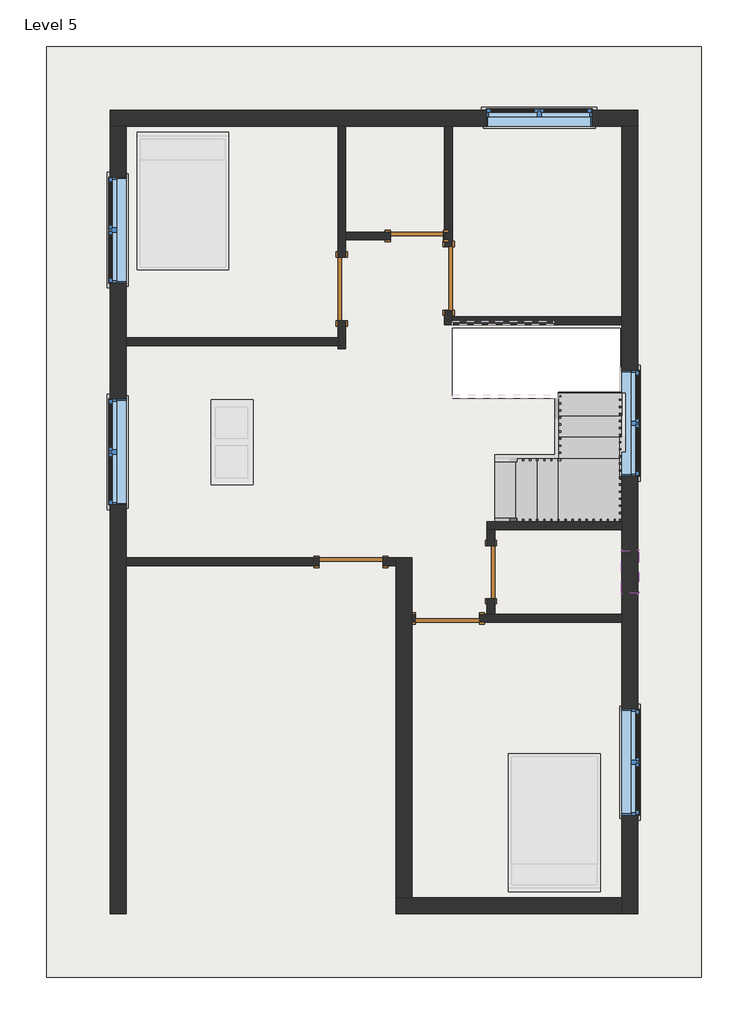
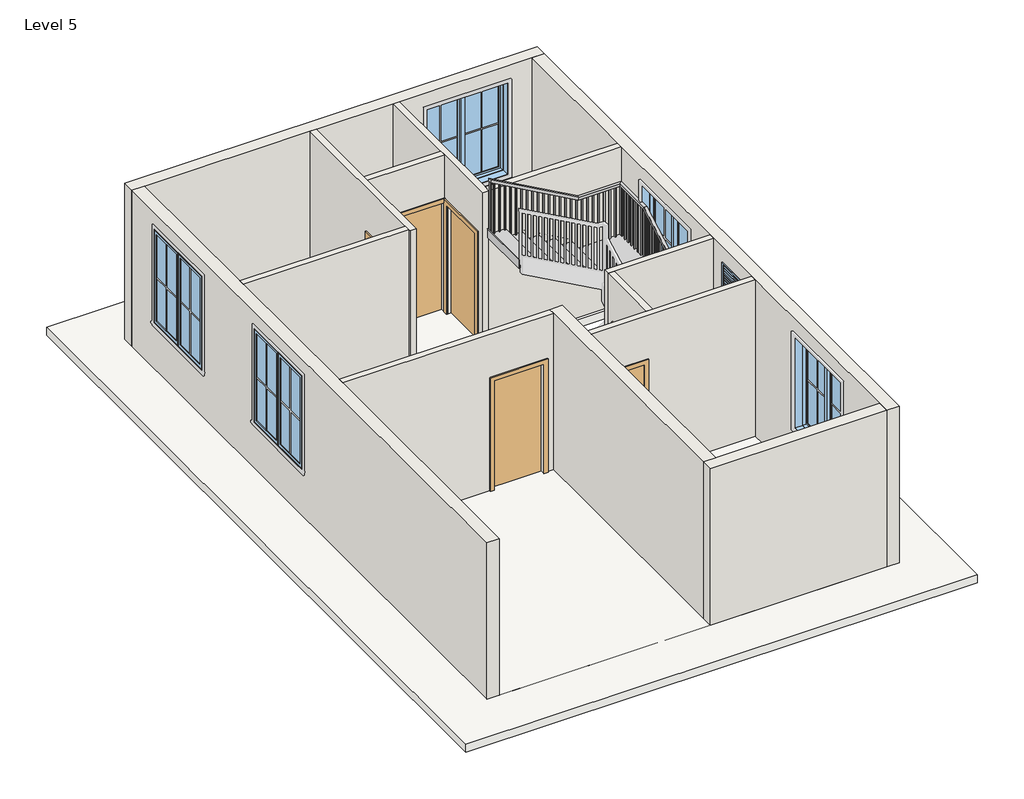
# One storey, part 1 of 2: 14 walls, 6 doors, 6 windows, 1 railing, 1 roof, 1 slab, 1 stair flight.
"""IFC4 building model written with IfcOpenShell, lengths in millimetres."""

from ifc_helpers import new_model, si_unit, frame, origin, place, context, project, spatial, polyline, outline, extrude, faceted_brep, transform, mapped, element, save
from components import door_214872d5, door_78caadf7, single_flush_door_3_e5f9f3c4, single_flush_door_3_305aa2a5, stair_flight_4ba9adf8, window_casement_double_win_5_f93960c7, window_f2d8fef0

model = new_model("IFC4")

# Units and contexts
model_context = context("Model", 3, world=origin())
ifc_project = project(units=[si_unit("LENGTHUNIT", "METRE", prefix="MILLI")], contexts=[model_context])

# Site, building, storey
site = spatial("IfcSite", under=ifc_project)
building = spatial("IfcBuilding", under=site)
storey = spatial("IfcBuildingStorey", under=building, Name="Level 5", Elevation=9601.2)

# Doors
placement = place(None, origin())
door_shape = door_214872d5(model_context)
element("IfcDoor", 1, ObjectType="Single-Flush : DOOR 2'6\"", at=placement, inside=storey, context=model_context, shape_type="MappedRepresentation", body=[
    mapped(door_shape, transform((-185.4325206, 3926.3629493, 9601.2), x_axis=(1.0, 0.0, 0.0), y_axis=(0.0, 1.0, 0.0), z_axis=(0.0, 0.0, 1.0))),
])
door_2_shape = door_78caadf7(model_context)
element("IfcDoor", 2, ObjectType="Single-Flush : DOOR 2'6\"", at=placement, inside=storey, context=model_context, shape_type="MappedRepresentation", body=[
    mapped(door_2_shape, transform((881.3674794, -905.9870507, 9601.2), x_axis=(0.0, 1.0, 0.0), y_axis=(-1.0, 0.0, 0.0), z_axis=(0.0, 0.0, 1.0))),
])
single_flush_door_3_shape = single_flush_door_3_e5f9f3c4(model_context)
element("IfcDoor", 3, ObjectType="Single-Flush : DOOR 3'", at=placement, inside=storey, context=model_context, shape_type="MappedRepresentation", body=[
    mapped(single_flush_door_3_shape, transform((271.7674794, 3316.7629493, 9601.2), x_axis=(0.0, -1.0, 0.0), y_axis=(1.0, 0.0, 0.0), z_axis=(0.0, 0.0, 1.0))),
])
element("IfcDoor", 4, ObjectType="Single-Flush : DOOR 3'", at=placement, inside=storey, context=model_context, shape_type="MappedRepresentation", body=[
    mapped(single_flush_door_3_shape, transform((255.8924794, -1572.7370507, 9601.2), x_axis=(-1.0, 0.0, 0.0), y_axis=(0.0, -1.0, 0.0), z_axis=(0.0, 0.0, 1.0))),
])
single_flush_door_3_2_shape = single_flush_door_3_305aa2a5(model_context)
element("IfcDoor", 5, ObjectType="Single-Flush : DOOR 3'", at=placement, inside=storey, context=model_context, shape_type="MappedRepresentation", body=[
    mapped(single_flush_door_3_2_shape, transform((-1264.9325206, 3164.3629493, 9601.2), x_axis=(0.0, -1.0, 0.0), y_axis=(1.0, 0.0, 0.0), z_axis=(0.0, 0.0, 1.0))),
])
element("IfcDoor", 6, ObjectType="Single-Flush : DOOR 3'6\"", at=placement, inside=storey, context=model_context, shape_type="MappedRepresentation", body=[
    mapped(single_flush_door_3_shape, transform((-1131.5825206, -759.9370507, 9601.2), x_axis=(1.0, 0.0, 0.0), y_axis=(0.0, 1.0, 0.0), z_axis=(0.0, 0.0, 1.0))),
])

# Railing
element("IfcRailing", 7, ObjectType="Handrail - Rectangular", at=placement, inside=storey, context=model_context, shape_type="SolidModel", body=[
    faceted_brep([(938.5174794, -131.2870507, 10684.9333333), (938.5174794, -131.2870507, 10626.820221), (938.5174794, -182.0870507, 10626.820221), (938.5174794, -182.0870507, 10684.9333333), (2005.3174794, -131.2870507, 11277.6), (2018.4810817, -131.2870507, 11226.8), (2018.4810817, -182.0870507, 11226.8), (2005.3174794, -182.0870507, 11277.6), (2716.5174794, -131.2870507, 11277.6), (2716.5174794, -131.2870507, 11226.8), (2767.3174794, -182.0870507, 11226.8), (2767.3174794, -182.0870507, 11277.6), (2716.5174794, 579.9129493, 11277.6), (2716.5174794, 593.0765516, 11226.8), (2767.3174794, 593.0765516, 11226.8), (2767.3174794, 579.9129493, 11277.6), (2716.5174794, 1843.5629493, 11979.6277778), (2716.5174794, 1856.7265516, 11928.8277778), (2767.3174794, 1856.7265516, 11928.8277778), (2767.3174794, 1843.5629493, 11979.6277778), (2716.5174794, 2599.2129493, 11979.6277778), (2716.5174794, 2599.2129493, 11928.8277778), (2767.3174794, 2650.0129493, 11928.8277778), (2767.3174794, 2650.0129493, 11979.6277778), (1960.8674794, 2599.2129493, 11979.6277778), (1947.7038772, 2599.2129493, 11928.8277778), (1947.7038772, 2650.0129493, 11928.8277778), (1960.8674794, 2650.0129493, 11979.6277778), (328.9174794, 2599.2129493, 12886.2666667), (328.9174794, 2650.0129493, 12886.2666667), (328.9174794, 2650.0129493, 12828.1535543), (328.9174794, 2599.2129493, 12828.1535543)], [[[0, 1, 2, 3]], [[1, 0, 4, 5]], [[2, 1, 5, 6]], [[3, 2, 6, 7]], [[0, 3, 7, 4]], [[5, 4, 8, 9]], [[6, 5, 9, 10]], [[7, 6, 10, 11]], [[4, 7, 11, 8]], [[9, 8, 12, 13]], [[10, 9, 13, 14]], [[11, 10, 14, 15]], [[8, 11, 15, 12]], [[13, 12, 16, 17]], [[14, 13, 17, 18]], [[15, 14, 18, 19]], [[12, 15, 19, 16]], [[17, 16, 20, 21]], [[18, 17, 21, 22]], [[19, 18, 22, 23]], [[16, 19, 23, 20]], [[21, 20, 24, 25]], [[22, 21, 25, 26]], [[23, 22, 26, 27]], [[20, 23, 27, 24]], [[28, 29, 30, 31]], [[25, 24, 28, 31]], [[26, 25, 31, 30]], [[27, 26, 30, 29]], [[24, 27, 29, 28]]]),
    extrude(outline(polyline([(12780.5285543, 414.6424794), (12791.1118876, 395.5924794), (11802.5333333, 395.5924794), (11802.5333333, 414.6424794), (12780.5285543, 414.6424794)])), frame((0.0, 2615.0879493, 0.0), z_axis=(0.0, 1.0, 0.0), x_axis=(0.0, 0.0, 1.0)), (0.0, 0.0, 1.0), 19.05),
    extrude(outline(polyline([(12724.0841099, 516.2424794), (12734.6674432, 497.1924794), (11802.5333333, 497.1924794), (11802.5333333, 516.2424794), (12724.0841099, 516.2424794)])), frame((0.0, 2615.0879493, 0.0), z_axis=(0.0, 1.0, 0.0), x_axis=(0.0, 0.0, 1.0)), (0.0, 0.0, 1.0), 19.05),
    extrude(outline(polyline([(12667.6396654, 617.8424794), (12678.2229988, 598.7924794), (11802.5333333, 598.7924794), (11802.5333333, 617.8424794), (12667.6396654, 617.8424794)])), frame((0.0, 2615.0879493, 0.0), z_axis=(0.0, 1.0, 0.0), x_axis=(0.0, 0.0, 1.0)), (0.0, 0.0, 1.0), 19.05),
    extrude(outline(polyline([(12611.195221, 719.4424794), (12621.7785543, 700.3924794), (11633.2, 700.3924794), (11633.2, 719.4424794), (12611.195221, 719.4424794)])), frame((0.0, 2615.0879493, 0.0), z_axis=(0.0, 1.0, 0.0), x_axis=(0.0, 0.0, 1.0)), (0.0, 0.0, 1.0), 19.05),
    extrude(outline(polyline([(12554.7507765, 821.0424794), (12565.3341099, 801.9924794), (11633.2, 801.9924794), (11633.2, 821.0424794), (12554.7507765, 821.0424794)])), frame((0.0, 2615.0879493, 0.0), z_axis=(0.0, 1.0, 0.0), x_axis=(0.0, 0.0, 1.0)), (0.0, 0.0, 1.0), 19.05),
    extrude(outline(polyline([(12498.3063321, 922.6424794), (12508.8896654, 903.5924794), (11633.2, 903.5924794), (11633.2, 922.6424794), (12498.3063321, 922.6424794)])), frame((0.0, 2615.0879493, 0.0), z_axis=(0.0, 1.0, 0.0), x_axis=(0.0, 0.0, 1.0)), (0.0, 0.0, 1.0), 19.05),
    extrude(outline(polyline([(12441.8618876, 1024.2424794), (12452.445221, 1005.1924794), (11463.8666667, 1005.1924794), (11463.8666667, 1024.2424794), (12441.8618876, 1024.2424794)])), frame((0.0, 2615.0879493, 0.0), z_axis=(0.0, 1.0, 0.0), x_axis=(0.0, 0.0, 1.0)), (0.0, 0.0, 1.0), 19.05),
    extrude(outline(polyline([(12385.4174432, 1125.8424794), (12396.0007765, 1106.7924794), (11463.8666667, 1106.7924794), (11463.8666667, 1125.8424794), (12385.4174432, 1125.8424794)])), frame((0.0, 2615.0879493, 0.0), z_axis=(0.0, 1.0, 0.0), x_axis=(0.0, 0.0, 1.0)), (0.0, 0.0, 1.0), 19.05),
    extrude(outline(polyline([(12328.9729988, 1227.4424794), (12339.5563321, 1208.3924794), (11463.8666667, 1208.3924794), (11463.8666667, 1227.4424794), (12328.9729988, 1227.4424794)])), frame((0.0, 2615.0879493, 0.0), z_axis=(0.0, 1.0, 0.0), x_axis=(0.0, 0.0, 1.0)), (0.0, 0.0, 1.0), 19.05),
    extrude(outline(polyline([(12272.5285543, 1329.0424794), (12283.1118876, 1309.9924794), (11294.5333333, 1309.9924794), (11294.5333333, 1329.0424794), (12272.5285543, 1329.0424794)])), frame((0.0, 2615.0879493, 0.0), z_axis=(0.0, 1.0, 0.0), x_axis=(0.0, 0.0, 1.0)), (0.0, 0.0, 1.0), 19.05),
    extrude(outline(polyline([(12216.0841099, 1430.6424794), (12226.6674432, 1411.5924794), (11294.5333333, 1411.5924794), (11294.5333333, 1430.6424794), (12216.0841099, 1430.6424794)])), frame((0.0, 2615.0879493, 0.0), z_axis=(0.0, 1.0, 0.0), x_axis=(0.0, 0.0, 1.0)), (0.0, 0.0, 1.0), 19.05),
    extrude(outline(polyline([(12159.6396654, 1532.2424794), (12170.2229988, 1513.1924794), (11294.5333333, 1513.1924794), (11294.5333333, 1532.2424794), (12159.6396654, 1532.2424794)])), frame((0.0, 2615.0879493, 0.0), z_axis=(0.0, 1.0, 0.0), x_axis=(0.0, 0.0, 1.0)), (0.0, 0.0, 1.0), 19.05),
    extrude(outline(polyline([(12103.195221, 1633.8424794), (12113.7785543, 1614.7924794), (11125.2, 1614.7924794), (11125.2, 1633.8424794), (12103.195221, 1633.8424794)])), frame((0.0, 2615.0879493, 0.0), z_axis=(0.0, 1.0, 0.0), x_axis=(0.0, 0.0, 1.0)), (0.0, 0.0, 1.0), 19.05),
    extrude(outline(polyline([(12046.7507765, 1735.4424794), (12057.3341099, 1716.3924794), (11125.2, 1716.3924794), (11125.2, 1735.4424794), (12046.7507765, 1735.4424794)])), frame((0.0, 2615.0879493, 0.0), z_axis=(0.0, 1.0, 0.0), x_axis=(0.0, 0.0, 1.0)), (0.0, 0.0, 1.0), 19.05),
    extrude(outline(polyline([(11990.3063321, 1837.0424794), (12000.8896654, 1817.9924794), (11125.2, 1817.9924794), (11125.2, 1837.0424794), (11990.3063321, 1837.0424794)])), frame((0.0, 2615.0879493, 0.0), z_axis=(0.0, 1.0, 0.0), x_axis=(0.0, 0.0, 1.0)), (0.0, 0.0, 1.0), 19.05),
    extrude(outline(polyline([(11933.8618876, 1938.6424794), (11944.445221, 1919.5924794), (10955.8666667, 1919.5924794), (10955.8666667, 1938.6424794), (11933.8618876, 1938.6424794)])), frame((0.0, 2615.0879493, 0.0), z_axis=(0.0, 1.0, 0.0), x_axis=(0.0, 0.0, 1.0)), (0.0, 0.0, 1.0), 19.05),
    extrude(outline(polyline([(2040.2424794, 2634.1379493), (2040.2424794, 2615.0879493), (2021.1924794, 2615.0879493), (2021.1924794, 2634.1379493), (2040.2424794, 2634.1379493)])), frame((0.0, 0.0, 10955.8666667), z_axis=(0.0, 0.0, 1.0), x_axis=(1.0, 0.0, 0.0)), (0.0, 0.0, 1.0), 972.9611111),
    extrude(outline(polyline([(2141.8424794, 2634.1379493), (2141.8424794, 2615.0879493), (2122.7924794, 2615.0879493), (2122.7924794, 2634.1379493), (2141.8424794, 2634.1379493)])), frame((0.0, 0.0, 10955.8666667), z_axis=(0.0, 0.0, 1.0), x_axis=(1.0, 0.0, 0.0)), (0.0, 0.0, 1.0), 972.9611111),
    extrude(outline(polyline([(2243.4424794, 2634.1379493), (2243.4424794, 2615.0879493), (2224.3924794, 2615.0879493), (2224.3924794, 2634.1379493), (2243.4424794, 2634.1379493)])), frame((0.0, 0.0, 10955.8666667), z_axis=(0.0, 0.0, 1.0), x_axis=(1.0, 0.0, 0.0)), (0.0, 0.0, 1.0), 972.9611111),
    extrude(outline(polyline([(2345.0424794, 2634.1379493), (2345.0424794, 2615.0879493), (2325.9924794, 2615.0879493), (2325.9924794, 2634.1379493), (2345.0424794, 2634.1379493)])), frame((0.0, 0.0, 10955.8666667), z_axis=(0.0, 0.0, 1.0), x_axis=(1.0, 0.0, 0.0)), (0.0, 0.0, 1.0), 972.9611111),
    extrude(outline(polyline([(2446.6424794, 2634.1379493), (2446.6424794, 2615.0879493), (2427.5924794, 2615.0879493), (2427.5924794, 2634.1379493), (2446.6424794, 2634.1379493)])), frame((0.0, 0.0, 10955.8666667), z_axis=(0.0, 0.0, 1.0), x_axis=(1.0, 0.0, 0.0)), (0.0, 0.0, 1.0), 972.9611111),
    extrude(outline(polyline([(2548.2424794, 2634.1379493), (2548.2424794, 2615.0879493), (2529.1924794, 2615.0879493), (2529.1924794, 2634.1379493), (2548.2424794, 2634.1379493)])), frame((0.0, 0.0, 10955.8666667), z_axis=(0.0, 0.0, 1.0), x_axis=(1.0, 0.0, 0.0)), (0.0, 0.0, 1.0), 972.9611111),
    extrude(outline(polyline([(2649.8424794, 2634.1379493), (2649.8424794, 2615.0879493), (2630.7924794, 2615.0879493), (2630.7924794, 2634.1379493), (2649.8424794, 2634.1379493)])), frame((0.0, 0.0, 10955.8666667), z_axis=(0.0, 0.0, 1.0), x_axis=(1.0, 0.0, 0.0)), (0.0, 0.0, 1.0), 972.9611111),
    extrude(outline(polyline([(2751.4424794, 2576.9879493), (2732.3924794, 2576.9879493), (2732.3924794, 2596.0379493), (2751.4424794, 2596.0379493), (2751.4424794, 2576.9879493)])), frame((0.0, 0.0, 10955.8666667), z_axis=(0.0, 0.0, 1.0), x_axis=(1.0, 0.0, 0.0)), (0.0, 0.0, 1.0), 972.9611111),
    extrude(outline(polyline([(2751.4424794, 2475.3879493), (2732.3924794, 2475.3879493), (2732.3924794, 2494.4379493), (2751.4424794, 2494.4379493), (2751.4424794, 2475.3879493)])), frame((0.0, 0.0, 10955.8666667), z_axis=(0.0, 0.0, 1.0), x_axis=(1.0, 0.0, 0.0)), (0.0, 0.0, 1.0), 972.9611111),
    extrude(outline(polyline([(2751.4424794, 2373.7879493), (2732.3924794, 2373.7879493), (2732.3924794, 2392.8379493), (2751.4424794, 2392.8379493), (2751.4424794, 2373.7879493)])), frame((0.0, 0.0, 10955.8666667), z_axis=(0.0, 0.0, 1.0), x_axis=(1.0, 0.0, 0.0)), (0.0, 0.0, 1.0), 972.9611111),
    extrude(outline(polyline([(2751.4424794, 2272.1879493), (2732.3924794, 2272.1879493), (2732.3924794, 2291.2379493), (2751.4424794, 2291.2379493), (2751.4424794, 2272.1879493)])), frame((0.0, 0.0, 10955.8666667), z_axis=(0.0, 0.0, 1.0), x_axis=(1.0, 0.0, 0.0)), (0.0, 0.0, 1.0), 972.9611111),
    extrude(outline(polyline([(2751.4424794, 2170.5879493), (2732.3924794, 2170.5879493), (2732.3924794, 2189.6379493), (2751.4424794, 2189.6379493), (2751.4424794, 2170.5879493)])), frame((0.0, 0.0, 10955.8666667), z_axis=(0.0, 0.0, 1.0), x_axis=(1.0, 0.0, 0.0)), (0.0, 0.0, 1.0), 972.9611111),
    extrude(outline(polyline([(2751.4424794, 2068.9879493), (2732.3924794, 2068.9879493), (2732.3924794, 2088.0379493), (2751.4424794, 2088.0379493), (2751.4424794, 2068.9879493)])), frame((0.0, 0.0, 10955.8666667), z_axis=(0.0, 0.0, 1.0), x_axis=(1.0, 0.0, 0.0)), (0.0, 0.0, 1.0), 972.9611111),
    extrude(outline(polyline([(2751.4424794, 1967.3879493), (2732.3924794, 1967.3879493), (2732.3924794, 1986.4379493), (2751.4424794, 1986.4379493), (2751.4424794, 1967.3879493)])), frame((0.0, 0.0, 10955.8666667), z_axis=(0.0, 0.0, 1.0), x_axis=(1.0, 0.0, 0.0)), (0.0, 0.0, 1.0), 972.9611111),
    extrude(outline(polyline([(2751.4424794, 1865.7879493), (2732.3924794, 1865.7879493), (2732.3924794, 1884.8379493), (2751.4424794, 1884.8379493), (2751.4424794, 1865.7879493)])), frame((0.0, 0.0, 10955.8666667), z_axis=(0.0, 0.0, 1.0), x_axis=(1.0, 0.0, 0.0)), (0.0, 0.0, 1.0), 972.9611111),
    extrude(outline(polyline([(1764.1879493, 11877.4174432), (1783.2379493, 11888.0007765), (1783.2379493, 10955.8666667), (1764.1879493, 10955.8666667), (1764.1879493, 11877.4174432)])), frame((2732.3924794, 0.0, 0.0), z_axis=(1.0, 0.0, 0.0), x_axis=(0.0, 1.0, 0.0)), (0.0, 0.0, 1.0), 19.05),
    extrude(outline(polyline([(1662.5879493, 11820.9729988), (1681.6379493, 11831.5563321), (1681.6379493, 10955.8666667), (1662.5879493, 10955.8666667), (1662.5879493, 11820.9729988)])), frame((2732.3924794, 0.0, 0.0), z_axis=(1.0, 0.0, 0.0), x_axis=(0.0, 1.0, 0.0)), (0.0, 0.0, 1.0), 19.05),
    extrude(outline(polyline([(1560.9879493, 11764.5285543), (1580.0379493, 11775.1118876), (1580.0379493, 10786.5333333), (1560.9879493, 10786.5333333), (1560.9879493, 11764.5285543)])), frame((2732.3924794, 0.0, 0.0), z_axis=(1.0, 0.0, 0.0), x_axis=(0.0, 1.0, 0.0)), (0.0, 0.0, 1.0), 19.05),
    extrude(outline(polyline([(1459.3879493, 11708.0841099), (1478.4379493, 11718.6674432), (1478.4379493, 10786.5333333), (1459.3879493, 10786.5333333), (1459.3879493, 11708.0841099)])), frame((2732.3924794, 0.0, 0.0), z_axis=(1.0, 0.0, 0.0), x_axis=(0.0, 1.0, 0.0)), (0.0, 0.0, 1.0), 19.05),
    extrude(outline(polyline([(1357.7879493, 11651.6396654), (1376.8379493, 11662.2229988), (1376.8379493, 10786.5333333), (1357.7879493, 10786.5333333), (1357.7879493, 11651.6396654)])), frame((2732.3924794, 0.0, 0.0), z_axis=(1.0, 0.0, 0.0), x_axis=(0.0, 1.0, 0.0)), (0.0, 0.0, 1.0), 19.05),
    extrude(outline(polyline([(1256.1879493, 11595.195221), (1275.2379493, 11605.7785543), (1275.2379493, 10617.2), (1256.1879493, 10617.2), (1256.1879493, 11595.195221)])), frame((2732.3924794, 0.0, 0.0), z_axis=(1.0, 0.0, 0.0), x_axis=(0.0, 1.0, 0.0)), (0.0, 0.0, 1.0), 19.05),
    extrude(outline(polyline([(1154.5879493, 11538.7507765), (1173.6379493, 11549.3341099), (1173.6379493, 10617.2), (1154.5879493, 10617.2), (1154.5879493, 11538.7507765)])), frame((2732.3924794, 0.0, 0.0), z_axis=(1.0, 0.0, 0.0), x_axis=(0.0, 1.0, 0.0)), (0.0, 0.0, 1.0), 19.05),
    extrude(outline(polyline([(1052.9879493, 11482.3063321), (1072.0379493, 11492.8896654), (1072.0379493, 10617.2), (1052.9879493, 10617.2), (1052.9879493, 11482.3063321)])), frame((2732.3924794, 0.0, 0.0), z_axis=(1.0, 0.0, 0.0), x_axis=(0.0, 1.0, 0.0)), (0.0, 0.0, 1.0), 19.05),
    extrude(outline(polyline([(951.3879493, 11425.8618876), (970.4379493, 11436.445221), (970.4379493, 10447.8666667), (951.3879493, 10447.8666667), (951.3879493, 11425.8618876)])), frame((2732.3924794, 0.0, 0.0), z_axis=(1.0, 0.0, 0.0), x_axis=(0.0, 1.0, 0.0)), (0.0, 0.0, 1.0), 19.05),
    extrude(outline(polyline([(849.7879493, 11369.4174432), (868.8379493, 11380.0007765), (868.8379493, 10447.8666667), (849.7879493, 10447.8666667), (849.7879493, 11369.4174432)])), frame((2732.3924794, 0.0, 0.0), z_axis=(1.0, 0.0, 0.0), x_axis=(0.0, 1.0, 0.0)), (0.0, 0.0, 1.0), 19.05),
    extrude(outline(polyline([(748.1879493, 11312.9729988), (767.2379493, 11323.5563321), (767.2379493, 10447.8666667), (748.1879493, 10447.8666667), (748.1879493, 11312.9729988)])), frame((2732.3924794, 0.0, 0.0), z_axis=(1.0, 0.0, 0.0), x_axis=(0.0, 1.0, 0.0)), (0.0, 0.0, 1.0), 19.05),
    extrude(outline(polyline([(646.5879493, 11256.5285543), (665.6379493, 11267.1118876), (665.6379493, 10278.5333333), (646.5879493, 10278.5333333), (646.5879493, 11256.5285543)])), frame((2732.3924794, 0.0, 0.0), z_axis=(1.0, 0.0, 0.0), x_axis=(0.0, 1.0, 0.0)), (0.0, 0.0, 1.0), 19.05),
    extrude(outline(polyline([(2751.4424794, 544.9879493), (2732.3924794, 544.9879493), (2732.3924794, 564.0379493), (2751.4424794, 564.0379493), (2751.4424794, 544.9879493)])), frame((0.0, 0.0, 10278.5333333), z_axis=(0.0, 0.0, 1.0), x_axis=(1.0, 0.0, 0.0)), (0.0, 0.0, 1.0), 948.2666667),
    extrude(outline(polyline([(2751.4424794, 443.3879493), (2732.3924794, 443.3879493), (2732.3924794, 462.4379493), (2751.4424794, 462.4379493), (2751.4424794, 443.3879493)])), frame((0.0, 0.0, 10278.5333333), z_axis=(0.0, 0.0, 1.0), x_axis=(1.0, 0.0, 0.0)), (0.0, 0.0, 1.0), 948.2666667),
    extrude(outline(polyline([(2751.4424794, 341.7879493), (2732.3924794, 341.7879493), (2732.3924794, 360.8379493), (2751.4424794, 360.8379493), (2751.4424794, 341.7879493)])), frame((0.0, 0.0, 10278.5333333), z_axis=(0.0, 0.0, 1.0), x_axis=(1.0, 0.0, 0.0)), (0.0, 0.0, 1.0), 948.2666667),
    extrude(outline(polyline([(2751.4424794, 240.1879493), (2732.3924794, 240.1879493), (2732.3924794, 259.2379493), (2751.4424794, 259.2379493), (2751.4424794, 240.1879493)])), frame((0.0, 0.0, 10278.5333333), z_axis=(0.0, 0.0, 1.0), x_axis=(1.0, 0.0, 0.0)), (0.0, 0.0, 1.0), 948.2666667),
    extrude(outline(polyline([(2751.4424794, 138.5879493), (2732.3924794, 138.5879493), (2732.3924794, 157.6379493), (2751.4424794, 157.6379493), (2751.4424794, 138.5879493)])), frame((0.0, 0.0, 10278.5333333), z_axis=(0.0, 0.0, 1.0), x_axis=(1.0, 0.0, 0.0)), (0.0, 0.0, 1.0), 948.2666667),
    extrude(outline(polyline([(2751.4424794, 36.9879493), (2732.3924794, 36.9879493), (2732.3924794, 56.0379493), (2751.4424794, 56.0379493), (2751.4424794, 36.9879493)])), frame((0.0, 0.0, 10278.5333333), z_axis=(0.0, 0.0, 1.0), x_axis=(1.0, 0.0, 0.0)), (0.0, 0.0, 1.0), 948.2666667),
    extrude(outline(polyline([(2751.4424794, -64.6120507), (2732.3924794, -64.6120507), (2732.3924794, -45.5620507), (2751.4424794, -45.5620507), (2751.4424794, -64.6120507)])), frame((0.0, 0.0, 10278.5333333), z_axis=(0.0, 0.0, 1.0), x_axis=(1.0, 0.0, 0.0)), (0.0, 0.0, 1.0), 948.2666667),
    extrude(outline(polyline([(2656.1924794, -166.2120507), (2656.1924794, -147.1620507), (2675.2424794, -147.1620507), (2675.2424794, -166.2120507), (2656.1924794, -166.2120507)])), frame((0.0, 0.0, 10278.5333333), z_axis=(0.0, 0.0, 1.0), x_axis=(1.0, 0.0, 0.0)), (0.0, 0.0, 1.0), 948.2666667),
    extrude(outline(polyline([(2554.5924794, -166.2120507), (2554.5924794, -147.1620507), (2573.6424794, -147.1620507), (2573.6424794, -166.2120507), (2554.5924794, -166.2120507)])), frame((0.0, 0.0, 10278.5333333), z_axis=(0.0, 0.0, 1.0), x_axis=(1.0, 0.0, 0.0)), (0.0, 0.0, 1.0), 948.2666667),
    extrude(outline(polyline([(2452.9924794, -166.2120507), (2452.9924794, -147.1620507), (2472.0424794, -147.1620507), (2472.0424794, -166.2120507), (2452.9924794, -166.2120507)])), frame((0.0, 0.0, 10278.5333333), z_axis=(0.0, 0.0, 1.0), x_axis=(1.0, 0.0, 0.0)), (0.0, 0.0, 1.0), 948.2666667),
    extrude(outline(polyline([(2351.3924794, -166.2120507), (2351.3924794, -147.1620507), (2370.4424794, -147.1620507), (2370.4424794, -166.2120507), (2351.3924794, -166.2120507)])), frame((0.0, 0.0, 10278.5333333), z_axis=(0.0, 0.0, 1.0), x_axis=(1.0, 0.0, 0.0)), (0.0, 0.0, 1.0), 948.2666667),
    extrude(outline(polyline([(2249.7924794, -166.2120507), (2249.7924794, -147.1620507), (2268.8424794, -147.1620507), (2268.8424794, -166.2120507), (2249.7924794, -166.2120507)])), frame((0.0, 0.0, 10278.5333333), z_axis=(0.0, 0.0, 1.0), x_axis=(1.0, 0.0, 0.0)), (0.0, 0.0, 1.0), 948.2666667),
    extrude(outline(polyline([(2148.1924794, -166.2120507), (2148.1924794, -147.1620507), (2167.2424794, -147.1620507), (2167.2424794, -166.2120507), (2148.1924794, -166.2120507)])), frame((0.0, 0.0, 10278.5333333), z_axis=(0.0, 0.0, 1.0), x_axis=(1.0, 0.0, 0.0)), (0.0, 0.0, 1.0), 948.2666667),
    extrude(outline(polyline([(2046.5924794, -166.2120507), (2046.5924794, -147.1620507), (2065.6424794, -147.1620507), (2065.6424794, -166.2120507), (2046.5924794, -166.2120507)])), frame((0.0, 0.0, 10278.5333333), z_axis=(0.0, 0.0, 1.0), x_axis=(1.0, 0.0, 0.0)), (0.0, 0.0, 1.0), 948.2666667),
    extrude(outline(polyline([(11196.5563321, 1964.0424794), (11185.9729988, 1944.9924794), (10278.5333333, 1944.9924794), (10278.5333333, 1964.0424794), (11196.5563321, 1964.0424794)])), frame((0.0, -166.2120507, 0.0), z_axis=(0.0, 1.0, 0.0), x_axis=(0.0, 0.0, 1.0)), (0.0, 0.0, 1.0), 19.05),
    extrude(outline(polyline([(11140.1118876, 1862.4424794), (11129.5285543, 1843.3924794), (10278.5333333, 1843.3924794), (10278.5333333, 1862.4424794), (11140.1118876, 1862.4424794)])), frame((0.0, -166.2120507, 0.0), z_axis=(0.0, 1.0, 0.0), x_axis=(0.0, 0.0, 1.0)), (0.0, 0.0, 1.0), 19.05),
    extrude(outline(polyline([(11083.6674432, 1760.8424794), (11073.0841099, 1741.7924794), (10109.2, 1741.7924794), (10109.2, 1760.8424794), (11083.6674432, 1760.8424794)])), frame((0.0, -166.2120507, 0.0), z_axis=(0.0, 1.0, 0.0), x_axis=(0.0, 0.0, 1.0)), (0.0, 0.0, 1.0), 19.05),
    extrude(outline(polyline([(11027.2229988, 1659.2424794), (11016.6396654, 1640.1924794), (10109.2, 1640.1924794), (10109.2, 1659.2424794), (11027.2229988, 1659.2424794)])), frame((0.0, -166.2120507, 0.0), z_axis=(0.0, 1.0, 0.0), x_axis=(0.0, 0.0, 1.0)), (0.0, 0.0, 1.0), 19.05),
    extrude(outline(polyline([(10970.7785543, 1557.6424794), (10960.195221, 1538.5924794), (10109.2, 1538.5924794), (10109.2, 1557.6424794), (10970.7785543, 1557.6424794)])), frame((0.0, -166.2120507, 0.0), z_axis=(0.0, 1.0, 0.0), x_axis=(0.0, 0.0, 1.0)), (0.0, 0.0, 1.0), 19.05),
    extrude(outline(polyline([(10914.3341099, 1456.0424794), (10903.7507765, 1436.9924794), (9939.8666667, 1436.9924794), (9939.8666667, 1456.0424794), (10914.3341099, 1456.0424794)])), frame((0.0, -166.2120507, 0.0), z_axis=(0.0, 1.0, 0.0), x_axis=(0.0, 0.0, 1.0)), (0.0, 0.0, 1.0), 19.05),
    extrude(outline(polyline([(10857.8896654, 1354.4424794), (10847.3063321, 1335.3924794), (9939.8666667, 1335.3924794), (9939.8666667, 1354.4424794), (10857.8896654, 1354.4424794)])), frame((0.0, -166.2120507, 0.0), z_axis=(0.0, 1.0, 0.0), x_axis=(0.0, 0.0, 1.0)), (0.0, 0.0, 1.0), 19.05),
    extrude(outline(polyline([(10801.445221, 1252.8424794), (10790.8618876, 1233.7924794), (9939.8666667, 1233.7924794), (9939.8666667, 1252.8424794), (10801.445221, 1252.8424794)])), frame((0.0, -166.2120507, 0.0), z_axis=(0.0, 1.0, 0.0), x_axis=(0.0, 0.0, 1.0)), (0.0, 0.0, 1.0), 19.05),
    extrude(outline(polyline([(10745.0007765, 1151.2424794), (10734.4174432, 1132.1924794), (9770.5333333, 1132.1924794), (9770.5333333, 1151.2424794), (10745.0007765, 1151.2424794)])), frame((0.0, -166.2120507, 0.0), z_axis=(0.0, 1.0, 0.0), x_axis=(0.0, 0.0, 1.0)), (0.0, 0.0, 1.0), 19.05),
    extrude(outline(polyline([(10688.5563321, 1049.6424794), (10677.9729988, 1030.5924794), (9770.5333333, 1030.5924794), (9770.5333333, 1049.6424794), (10688.5563321, 1049.6424794)])), frame((0.0, -166.2120507, 0.0), z_axis=(0.0, 1.0, 0.0), x_axis=(0.0, 0.0, 1.0)), (0.0, 0.0, 1.0), 19.05),
    extrude(outline(polyline([(2751.4424794, 2615.0879493), (2732.3924794, 2615.0879493), (2732.3924794, 2634.1379493), (2751.4424794, 2634.1379493), (2751.4424794, 2615.0879493)])), frame((0.0, 0.0, 10955.8666667), z_axis=(0.0, 0.0, 1.0), x_axis=(1.0, 0.0, 0.0)), (0.0, 0.0, 1.0), 972.9611111),
    extrude(outline(polyline([(2732.3924794, -166.2120507), (2732.3924794, -147.1620507), (2751.4424794, -147.1620507), (2751.4424794, -166.2120507), (2732.3924794, -166.2120507)])), frame((0.0, 0.0, 10278.5333333), z_axis=(0.0, 0.0, 1.0), x_axis=(1.0, 0.0, 0.0)), (0.0, 0.0, 1.0), 948.2666667),
    extrude(outline(polyline([(12817.570221, 347.9674794), (12828.1535543, 328.9174794), (11802.5333333, 328.9174794), (11802.5333333, 347.9674794), (12817.570221, 347.9674794)])), frame((0.0, 2615.0879493, 0.0), z_axis=(0.0, 1.0, 0.0), x_axis=(0.0, 0.0, 1.0)), (0.0, 0.0, 1.0), 19.05),
    extrude(outline(polyline([(10637.4035543, 957.5674794), (10626.820221, 938.5174794), (9770.5333333, 938.5174794), (9770.5333333, 957.5674794), (10637.4035543, 957.5674794)])), frame((0.0, -166.2120507, 0.0), z_axis=(0.0, 1.0, 0.0), x_axis=(0.0, 0.0, 1.0)), (0.0, 0.0, 1.0), 19.05),
])

# Roof
element("IfcRoof", 8, ObjectType="ROOF 6\"", at=placement, inside=storey, context=model_context, shape_type="SweptSolid", body=[
    extrude(outline(polyline([(-5513.0825206, 6650.5129493), (3910.3174794, 6650.5129493), (3910.3174794, -6735.2870507), (-5513.0825206, -6735.2870507), (-5513.0825206, 6650.5129493)]), holes=[polyline([(2741.9174794, -156.6870507), (2741.9174794, 2599.2129493), (328.9174794, 2599.2129493), (328.9174794, 1595.9129493), (1802.1174794, 1595.9129493), (1802.1174794, 706.9129493), (1040.1174794, 706.9129493), (1040.1174794, -156.6870507), (2741.9174794, -156.6870507)])]), frame((0.0, 0.0, 9448.8), z_axis=(0.0, 0.0, 1.0), x_axis=(1.0, 0.0, 0.0)), (0.0, 0.0, 1.0), 152.4),
])

# Slab
element("IfcSlab", 9, ObjectType="FLOOR 6\"", at=placement, inside=storey, context=model_context, shape_type="SweptSolid", body=[
    extrude(outline(polyline([(2995.9174794, 5736.1129493), (2995.9174794, -5820.8870507), (-4598.6825206, -5820.8870507), (-4598.6825206, 5736.1129493), (2995.9174794, 5736.1129493)]), holes=[polyline([(2741.9174794, -156.6870507), (2741.9174794, 2599.2129493), (328.9174794, 2599.2129493), (328.9174794, 1595.9129493), (1802.1174794, 1595.9129493), (1802.1174794, 706.9129493), (1040.1174794, 706.9129493), (1040.1174794, -156.6870507), (2741.9174794, -156.6870507)])]), frame((0.0, 0.0, 9448.8), z_axis=(0.0, 0.0, 1.0), x_axis=(1.0, 0.0, 0.0)), (0.0, 0.0, 1.0), 152.4),
])

# Stair flight
stair_flight_shape = stair_flight_4ba9adf8(model_context)
element("IfcStairFlight", 10, ObjectType="2\" Tread 1\" Nosing 1/4\" Riser", at=placement, inside=storey, context=model_context, shape_type="MappedRepresentation", body=[
    mapped(stair_flight_shape, transform((0.0, 0.0, 0.0), x_axis=(1.0, 0.0, 0.0), y_axis=(0.0, 1.0, 0.0), z_axis=(0.0, 0.0, 1.0))),
])

# Walls
element("IfcWall", 11, at=placement, inside=storey, context=model_context, shape_type="Brep", body=[
    faceted_brep([(-1322.0825206, 2707.1629493, 11734.8), (-1322.0825206, 2707.1629493, 9601.2), (-1322.0825206, 2459.5129493, 9601.2), (-1322.0825206, 2345.2129493, 9601.2), (-1322.0825206, 2307.1129493, 9601.2), (-1322.0825206, 2307.1129493, 12649.2), (-1322.0825206, 2345.2129493, 12649.2), (-1322.0825206, 2459.5129493, 12649.2), (-1322.0825206, 5507.5129493, 12649.2), (-1322.0825206, 5507.5129493, 9601.2), (-1322.0825206, 3621.5629493, 9601.2), (-1322.0825206, 3621.5629493, 11734.8), (-1207.7825206, 2307.1129493, 9601.2), (-1207.7825206, 2707.1629493, 9601.2), (-1207.7825206, 2707.1629493, 11734.8), (-1207.7825206, 3621.5629493, 11734.8), (-1207.7825206, 3621.5629493, 9601.2), (-1207.7825206, 3869.2129493, 9601.2), (-1207.7825206, 3983.5129493, 9601.2), (-1207.7825206, 5507.5129493, 9601.2), (-1207.7825206, 5507.5129493, 12649.2), (-1207.7825206, 3983.5129493, 12649.2), (-1207.7825206, 3869.2129493, 12649.2), (-1207.7825206, 2307.1129493, 12649.2)], [[[0, 1, 2, 3, 4, 5, 6, 7, 8, 9, 10, 11]], [[12, 13, 14, 15, 16, 17, 18, 19, 20, 21, 22, 23]], [[10, 9, 19, 18, 17, 16]], [[4, 3, 2, 1, 13, 12]], [[5, 4, 12, 23]], [[9, 8, 20, 19]], [[14, 13, 1, 0]], [[15, 14, 0, 11]], [[16, 15, 11, 10]], [[8, 7, 6, 5, 23, 22, 21, 20]]]),
])
element("IfcWall", 12, at=placement, inside=storey, context=model_context, shape_type="SweptSolid", body=[
    extrude(outline(polyline([(-1322.0825206, 2345.2129493), (-4370.0825206, 2345.2129493), (-4370.0825206, 2459.5129493), (-1322.0825206, 2459.5129493), (-1322.0825206, 2345.2129493)])), frame((0.0, 0.0, 9601.2), z_axis=(0.0, 0.0, 1.0), x_axis=(1.0, 0.0, 0.0)), (0.0, 0.0, 1.0), 3048.0),
])
element("IfcWall", 13, at=placement, inside=storey, context=model_context, shape_type="SweptSolid", body=[
    extrude(outline(polyline([(11734.8, 195.5674794), (9601.2, 195.5674794), (9601.2, 214.6174794), (12649.2, 214.6174794), (12649.2, -1207.7825206), (9601.2, -1207.7825206), (9601.2, -566.4325206), (11734.8, -566.4325206), (11734.8, 195.5674794)])), frame((0.0, 3869.2129493, 0.0), z_axis=(0.0, 1.0, 0.0), x_axis=(0.0, 0.0, 1.0)), (0.0, 0.0, 1.0), 114.3),
])
element("IfcWall", 14, at=placement, inside=storey, context=model_context, shape_type="Brep", body=[
    faceted_brep([(214.6174794, 2859.5629493, 11734.8), (214.6174794, 2859.5629493, 9601.2), (214.6174794, 2650.0129493, 9601.2), (214.6174794, 2650.0129493, 12649.2), (214.6174794, 3869.2129493, 12649.2), (214.6174794, 3983.5129493, 12649.2), (214.6174794, 5507.5129493, 12649.2), (214.6174794, 5507.5129493, 9601.2), (214.6174794, 3983.5129493, 9601.2), (214.6174794, 3869.2129493, 9601.2), (214.6174794, 3773.9629493, 9601.2), (214.6174794, 3773.9629493, 11734.8), (328.9174794, 2650.0129493, 9601.2), (328.9174794, 2764.3129493, 9601.2), (328.9174794, 2859.5629493, 9601.2), (328.9174794, 2859.5629493, 11734.8), (328.9174794, 3773.9629493, 11734.8), (328.9174794, 3773.9629493, 9601.2), (328.9174794, 5507.5129493, 9601.2), (328.9174794, 5507.5129493, 12649.2), (328.9174794, 2764.3129493, 12649.2), (328.9174794, 2650.0129493, 12649.2)], [[[0, 1, 2, 3, 4, 5, 6, 7, 8, 9, 10, 11]], [[12, 13, 14, 15, 16, 17, 18, 19, 20, 21]], [[2, 1, 14, 13, 12]], [[10, 9, 8, 7, 18, 17]], [[7, 6, 19, 18]], [[3, 2, 12, 21]], [[15, 14, 1, 0]], [[16, 15, 0, 11]], [[17, 16, 11, 10]], [[6, 5, 4, 3, 21, 20, 19]]]),
])
element("IfcWall", 15, at=placement, inside=storey, context=model_context, shape_type="SweptSolid", body=[
    extrude(outline(polyline([(2767.3174794, 2650.0129493), (328.9174794, 2650.0129493), (328.9174794, 2764.3129493), (2767.3174794, 2764.3129493), (2767.3174794, 2650.0129493)])), frame((0.0, 0.0, 9601.2), z_axis=(0.0, 0.0, 1.0), x_axis=(1.0, 0.0, 0.0)), (0.0, 0.0, 1.0), 3048.0),
])
element("IfcWall", 16, at=placement, inside=storey, context=model_context, shape_type="Brep", body=[
    faceted_brep([(2767.3174794, -182.0870507, 9601.2), (824.2174794, -182.0870507, 9601.2), (824.2174794, -182.0870507, 12649.2), (2767.3174794, -182.0870507, 12649.2), (2767.3174794, -296.3870507, 9601.2), (2767.3174794, -296.3870507, 12649.2), (938.5174794, -296.3870507, 12649.2), (824.2174794, -296.3870507, 12649.2), (824.2174794, -296.3870507, 9601.2), (938.5174794, -296.3870507, 9601.2)], [[[0, 1, 2, 3]], [[4, 5, 6, 7, 8, 9]], [[1, 0, 4, 9, 8]], [[0, 3, 5, 4]], [[2, 1, 8, 7]], [[3, 2, 7, 6, 5]]]),
])
element("IfcWall", 17, at=placement, inside=storey, context=model_context, shape_type="SweptSolid", body=[
    extrude(outline(polyline([(-296.3870507, 9601.2), (-524.9870507, 9601.2), (-524.9870507, 11734.8), (-1286.9870507, 11734.8), (-1286.9870507, 9601.2), (-1515.5870507, 9601.2), (-1515.5870507, 12649.2), (-296.3870507, 12649.2), (-296.3870507, 9601.2)])), frame((824.2174794, 0.0, 0.0), z_axis=(1.0, 0.0, 0.0), x_axis=(0.0, 1.0, 0.0)), (0.0, 0.0, 1.0), 114.3),
])
element("IfcWall", 18, at=placement, inside=storey, context=model_context, shape_type="Brep", body=[
    faceted_brep([(-201.3075206, -1515.5870507, 11734.8), (-201.3075206, -1515.5870507, 9601.2), (-255.2825206, -1515.5870507, 9601.2), (-255.2825206, -1515.5870507, 12649.2), (824.2174794, -1515.5870507, 12649.2), (938.5174794, -1515.5870507, 12649.2), (2767.3174794, -1515.5870507, 12649.2), (2767.3174794, -1515.5870507, 9601.2), (938.5174794, -1515.5870507, 9601.2), (824.2174794, -1515.5870507, 9601.2), (713.0924794, -1515.5870507, 9601.2), (713.0924794, -1515.5870507, 11734.8), (-255.2825206, -1629.8870507, 9601.2), (-201.3075206, -1629.8870507, 9601.2), (-201.3075206, -1629.8870507, 11734.8), (713.0924794, -1629.8870507, 11734.8), (713.0924794, -1629.8870507, 9601.2), (2767.3174794, -1629.8870507, 9601.2), (2767.3174794, -1629.8870507, 12649.2), (-255.2825206, -1629.8870507, 12649.2)], [[[0, 1, 2, 3, 4, 5, 6, 7, 8, 9, 10, 11]], [[12, 13, 14, 15, 16, 17, 18, 19]], [[2, 1, 13, 12]], [[10, 9, 8, 7, 17, 16]], [[7, 6, 18, 17]], [[3, 2, 12, 19]], [[14, 13, 1, 0]], [[15, 14, 0, 11]], [[16, 15, 11, 10]], [[6, 5, 4, 3, 19, 18]]]),
])
element("IfcWall", 19, at=placement, inside=storey, context=model_context, shape_type="SweptSolid", body=[
    extrude(outline(polyline([(11734.8, -674.3825206), (9601.2, -674.3825206), (9601.2, -483.8825206), (12649.2, -483.8825206), (12649.2, -4370.0825206), (9601.2, -4370.0825206), (9601.2, -1588.7825206), (11734.8, -1588.7825206), (11734.8, -674.3825206)])), frame((0.0, -817.0870507, 0.0), z_axis=(0.0, 1.0, 0.0), x_axis=(0.0, 0.0, 1.0)), (0.0, 0.0, 1.0), 114.3),
])
element("IfcWall", 20, ObjectType="WALL 9\"", at=placement, inside=storey, context=model_context, shape_type="Brep", body=[
    faceted_brep([(-4598.6825206, 5507.5129493, 9601.2), (-4370.0825206, 5507.5129493, 9601.2), (-1322.0825206, 5507.5129493, 9601.2), (-1207.7825206, 5507.5129493, 9601.2), (214.6174794, 5507.5129493, 9601.2), (328.9174794, 5507.5129493, 9601.2), (2767.3174794, 5507.5129493, 9601.2), (2995.9174794, 5507.5129493, 9601.2), (2995.9174794, 5507.5129493, 12649.2), (2767.3174794, 5507.5129493, 12649.2), (328.9174794, 5507.5129493, 12649.2), (214.6174794, 5507.5129493, 12649.2), (-1207.7825206, 5507.5129493, 12649.2), (-1322.0825206, 5507.5129493, 12649.2), (-4370.0825206, 5507.5129493, 12649.2), (-4598.6825206, 5507.5129493, 12649.2), (2338.6924794, 5507.5129493, 12344.4), (2338.6924794, 5507.5129493, 10515.6), (814.6924794, 5507.5129493, 10515.6), (814.6924794, 5507.5129493, 12344.4), (-4598.6825206, 5736.1129493, 9601.2), (-4598.6825206, 5736.1129493, 12649.2), (2995.9174794, 5736.1129493, 12649.2), (2995.9174794, 5736.1129493, 9601.2), (2338.6924794, 5736.1129493, 12344.4), (814.6924794, 5736.1129493, 12344.4), (814.6924794, 5736.1129493, 10515.6), (2338.6924794, 5736.1129493, 10515.6)], [[[0, 1, 2, 3, 4, 5, 6, 7, 8, 9, 10, 11, 12, 13, 14, 15], [16, 17, 18, 19]], [[20, 21, 22, 23], [24, 25, 26, 27]], [[7, 6, 5, 4, 3, 2, 1, 0, 20, 23]], [[8, 7, 23, 22]], [[0, 15, 21, 20]], [[17, 16, 24, 27]], [[18, 17, 27, 26]], [[19, 18, 26, 25]], [[16, 19, 25, 24]], [[15, 14, 13, 12, 11, 10, 9, 8, 22, 21]]]),
])
element("IfcWall", 21, ObjectType="WALL 9\"", at=placement, inside=storey, context=model_context, shape_type="Brep", body=[
    faceted_brep([(2767.3174794, 5507.5129493, 9601.2), (2767.3174794, 2764.3129493, 9601.2), (2767.3174794, 2650.0129493, 9601.2), (2767.3174794, -182.0870507, 9601.2), (2767.3174794, -296.3870507, 9601.2), (2767.3174794, -1515.5870507, 9601.2), (2767.3174794, -1629.8870507, 9601.2), (2767.3174794, -5592.2870507, 9601.2), (2767.3174794, -5820.8870507, 9601.2), (2767.3174794, -5820.8870507, 12649.2), (2767.3174794, -5592.2870507, 12649.2), (2767.3174794, -1629.8870507, 12649.2), (2767.3174794, -1515.5870507, 12649.2), (2767.3174794, -296.3870507, 12649.2), (2767.3174794, -182.0870507, 12649.2), (2767.3174794, 2650.0129493, 12649.2), (2767.3174794, 2764.3129493, 12649.2), (2767.3174794, 5507.5129493, 12649.2), (2767.3174794, 471.9629493, 12344.4), (2767.3174794, 471.9629493, 10515.6), (2767.3174794, 1995.9629493, 10515.6), (2767.3174794, 1995.9629493, 12344.4), (2767.3174794, -4401.6620507, 12344.4), (2767.3174794, -4401.6620507, 10515.6), (2767.3174794, -2877.6620507, 10515.6), (2767.3174794, -2877.6620507, 12344.4), (2767.3174794, -1210.7870507, 12344.4), (2767.3174794, -1210.7870507, 11734.8), (2767.3174794, -601.1870507, 11734.8), (2767.3174794, -601.1870507, 12344.4), (2995.9174794, 5507.5129493, 9601.2), (2995.9174794, 5507.5129493, 12649.2), (2995.9174794, -5820.8870507, 12649.2), (2995.9174794, -5820.8870507, 9601.2), (2995.9174794, 471.9629493, 12344.4), (2995.9174794, 1995.9629493, 12344.4), (2995.9174794, 1995.9629493, 10515.6), (2995.9174794, 471.9629493, 10515.6), (2995.9174794, -4401.6620507, 12344.4), (2995.9174794, -2877.6620507, 12344.4), (2995.9174794, -2877.6620507, 10515.6), (2995.9174794, -4401.6620507, 10515.6), (2995.9174794, -1210.7870507, 12344.4), (2995.9174794, -601.1870507, 12344.4), (2995.9174794, -601.1870507, 11734.8), (2995.9174794, -1210.7870507, 11734.8)], [[[0, 1, 2, 3, 4, 5, 6, 7, 8, 9, 10, 11, 12, 13, 14, 15, 16, 17], [18, 19, 20, 21], [22, 23, 24, 25], [26, 27, 28, 29]], [[30, 31, 32, 33], [34, 35, 36, 37], [38, 39, 40, 41], [42, 43, 44, 45]], [[8, 7, 6, 5, 4, 3, 2, 1, 0, 30, 33]], [[0, 17, 31, 30]], [[9, 8, 33, 32]], [[19, 18, 34, 37]], [[20, 19, 37, 36]], [[21, 20, 36, 35]], [[18, 21, 35, 34]], [[23, 22, 38, 41]], [[24, 23, 41, 40]], [[25, 24, 40, 39]], [[22, 25, 39, 38]], [[27, 26, 42, 45]], [[28, 27, 45, 44]], [[29, 28, 44, 43]], [[26, 29, 43, 42]], [[17, 16, 15, 14, 13, 12, 11, 10, 9, 32, 31]]]),
])
element("IfcWall", 22, ObjectType="WALL 9\"", at=placement, inside=storey, context=model_context, shape_type="Brep", body=[
    faceted_brep([(2767.3174794, -5592.2870507, 9601.2), (-255.2825206, -5592.2870507, 9601.2), (-483.8825206, -5592.2870507, 9601.2), (-483.8825206, -5592.2870507, 12649.2), (-255.2825206, -5592.2870507, 12649.2), (2767.3174794, -5592.2870507, 12649.2), (2767.3174794, -5820.8870507, 9601.2), (2767.3174794, -5820.8870507, 12649.2), (-483.8825206, -5820.8870507, 12649.2), (-483.8825206, -5820.8870507, 9601.2)], [[[0, 1, 2, 3, 4, 5]], [[6, 7, 8, 9]], [[2, 1, 0, 6, 9]], [[0, 5, 7, 6]], [[3, 2, 9, 8]], [[5, 4, 3, 8, 7]]]),
])
element("IfcWall", 23, ObjectType="WALL 9\"", at=placement, inside=storey, context=model_context, shape_type="Brep", body=[
    faceted_brep([(-255.2825206, -5592.2870507, 9601.2), (-255.2825206, -1629.8870507, 9601.2), (-255.2825206, -1515.5870507, 9601.2), (-255.2825206, -702.7870507, 9601.2), (-255.2825206, -702.7870507, 12649.2), (-255.2825206, -1515.5870507, 12649.2), (-255.2825206, -1629.8870507, 12649.2), (-255.2825206, -5592.2870507, 12649.2), (-483.8825206, -5592.2870507, 9601.2), (-483.8825206, -5592.2870507, 12649.2), (-483.8825206, -817.0870507, 12649.2), (-483.8825206, -702.7870507, 12649.2), (-483.8825206, -702.7870507, 9601.2), (-483.8825206, -817.0870507, 9601.2)], [[[0, 1, 2, 3, 4, 5, 6, 7]], [[8, 9, 10, 11, 12, 13]], [[3, 2, 1, 0, 8, 13, 12]], [[0, 7, 9, 8]], [[4, 3, 12, 11]], [[7, 6, 5, 4, 11, 10, 9]]]),
])
element("IfcWall", 24, ObjectType="WALL 9\"", at=placement, inside=storey, context=model_context, shape_type="Brep", body=[
    faceted_brep([(-4370.0825206, -5820.8870507, 9601.2), (-4370.0825206, -817.0870507, 9601.2), (-4370.0825206, -702.7870507, 9601.2), (-4370.0825206, 2345.2129493, 9601.2), (-4370.0825206, 2459.5129493, 9601.2), (-4370.0825206, 5507.5129493, 9601.2), (-4370.0825206, 5507.5129493, 12649.2), (-4370.0825206, 2459.5129493, 12649.2), (-4370.0825206, 2345.2129493, 12649.2), (-4370.0825206, -702.7870507, 12649.2), (-4370.0825206, -817.0870507, 12649.2), (-4370.0825206, -5820.8870507, 12649.2), (-4370.0825206, 1583.2129493, 12344.4), (-4370.0825206, 1583.2129493, 10515.6), (-4370.0825206, 59.2129493, 10515.6), (-4370.0825206, 59.2129493, 12344.4), (-4370.0825206, 4774.0879493, 12344.4), (-4370.0825206, 4774.0879493, 10515.6), (-4370.0825206, 3250.0879493, 10515.6), (-4370.0825206, 3250.0879493, 12344.4), (-4598.6825206, -5820.8870507, 9601.2), (-4598.6825206, -5820.8870507, 12649.2), (-4598.6825206, 5507.5129493, 12649.2), (-4598.6825206, 5507.5129493, 9601.2), (-4598.6825206, 1583.2129493, 12344.4), (-4598.6825206, 59.2129493, 12344.4), (-4598.6825206, 59.2129493, 10515.6), (-4598.6825206, 1583.2129493, 10515.6), (-4598.6825206, 4774.0879493, 12344.4), (-4598.6825206, 3250.0879493, 12344.4), (-4598.6825206, 3250.0879493, 10515.6), (-4598.6825206, 4774.0879493, 10515.6)], [[[0, 1, 2, 3, 4, 5, 6, 7, 8, 9, 10, 11], [12, 13, 14, 15], [16, 17, 18, 19]], [[20, 21, 22, 23], [24, 25, 26, 27], [28, 29, 30, 31]], [[5, 4, 3, 2, 1, 0, 20, 23]], [[0, 11, 21, 20]], [[6, 5, 23, 22]], [[13, 12, 24, 27]], [[14, 13, 27, 26]], [[15, 14, 26, 25]], [[12, 15, 25, 24]], [[17, 16, 28, 31]], [[18, 17, 31, 30]], [[19, 18, 30, 29]], [[16, 19, 29, 28]], [[11, 10, 9, 8, 7, 6, 22, 21]]]),
])

# Windows
window_casement_double_win_5_shape = window_casement_double_win_5_f93960c7(model_context)
element("IfcWindow", 25, ObjectType="Window-Casement-Double : WIN 5'", at=placement, inside=storey, context=model_context, shape_type="MappedRepresentation", body=[
    mapped(window_casement_double_win_5_shape, transform((-4484.3825206, 821.2129493, 9601.2), x_axis=(0.0, 1.0, 0.0), y_axis=(-1.0, 0.0, 0.0), z_axis=(0.0, 0.0, 1.0))),
])
element("IfcWindow", 26, ObjectType="Window-Casement-Double : WIN 5'", at=placement, inside=storey, context=model_context, shape_type="MappedRepresentation", body=[
    mapped(window_casement_double_win_5_shape, transform((-4484.3825206, 4012.0879493, 9601.2), x_axis=(0.0, 1.0, 0.0), y_axis=(-1.0, 0.0, 0.0), z_axis=(0.0, 0.0, 1.0))),
])
element("IfcWindow", 27, ObjectType="Window-Casement-Double : WIN 5'", at=placement, inside=storey, context=model_context, shape_type="MappedRepresentation", body=[
    mapped(window_casement_double_win_5_shape, transform((1576.6924794, 5621.8129493, 9601.2), x_axis=(1.0, 0.0, 0.0), y_axis=(0.0, 1.0, 0.0), z_axis=(0.0, 0.0, 1.0))),
])
element("IfcWindow", 28, ObjectType="Window-Casement-Double : WIN 5'", at=placement, inside=storey, context=model_context, shape_type="MappedRepresentation", body=[
    mapped(window_casement_double_win_5_shape, transform((2881.6174794, 1233.9629493, 9601.2), x_axis=(0.0, -1.0, 0.0), y_axis=(1.0, 0.0, 0.0), z_axis=(0.0, 0.0, 1.0))),
])
element("IfcWindow", 29, ObjectType="Window-Casement-Double : WIN 5'", at=placement, inside=storey, context=model_context, shape_type="MappedRepresentation", body=[
    mapped(window_casement_double_win_5_shape, transform((2881.6174794, -3639.6620507, 9601.2), x_axis=(0.0, -1.0, 0.0), y_axis=(1.0, 0.0, 0.0), z_axis=(0.0, 0.0, 1.0))),
])
window_shape = window_f2d8fef0(model_context)
element("IfcWindow", 30, ObjectType="Window-Louvers : 24\" x 24\"", at=placement, inside=storey, context=model_context, shape_type="MappedRepresentation", body=[
    mapped(window_shape, transform((2875.2674794, -905.9870507, 10820.4), x_axis=(0.0, 1.0, 0.0), y_axis=(-1.0, 0.0, 0.0), z_axis=(0.0, 0.0, 1.0))),
])

save(model, "model.ifc")

# Revit data of these elements
# Type "Single-Flush : DOOR 2'6\""
#   Type Mark = "10"
#   Construction Type Id = "MDOOR"
#   Assembly Code = "C1020"
#   Analytic Construction = "Metal"
#   Thickness = 0' - 2"
#   Heat Transfer Coefficient (U) = 0.651978 BTU/(h·ft²·°F)
#   Height = 7' - 0"
#   Trim Projection Ext = 0' - 1"
#   Trim Projection Int = 0' - 1"
#   Trim Width = 0' - 3"
#   Width = 2' - 6"
#   Define Thermal Properties by = 1
#   Door Material = Door - Panel
#   Frame Material = Door - Frame
#   Visual Light Transmittance = 0
#   Solar Heat Gain Coefficient = 0
#   Function = (empty or 0)
#   Wall Closure = (empty or 0)
# Type "Single-Flush : DOOR 3'"
#   Type Mark = "9"
#   Construction Type Id = "MDOOR"
#   Assembly Code = "C1020"
#   Analytic Construction = "Metal"
#   Thickness = 0' - 2"
#   Heat Transfer Coefficient (U) = 0.651978 BTU/(h·ft²·°F)
#   Height = 7' - 0"
#   Trim Projection Ext = 0' - 1"
#   Trim Projection Int = 0' - 1"
#   Trim Width = 0' - 3"
#   Width = 3' - 0"
#   Define Thermal Properties by = 1
#   Door Material = Door - Panel
#   Frame Material = Door - Frame
#   Visual Light Transmittance = 0
#   Solar Heat Gain Coefficient = 0
#   Function = (empty or 0)
#   Wall Closure = (empty or 0)
# Type "Single-Flush : DOOR 3'6\""
#   Type Mark = "8"
#   Construction Type Id = "MDOOR"
#   Assembly Code = "C1020"
#   Analytic Construction = "Metal"
#   Thickness = 0' - 2"
#   Heat Transfer Coefficient (U) = 0.651978 BTU/(h·ft²·°F)
#   Height = 7' - 0"
#   Trim Projection Ext = 0' - 1"
#   Trim Projection Int = 0' - 1"
#   Trim Width = 0' - 3"
#   Width = 3' - 0"
#   Define Thermal Properties by = 1
#   Door Material = Door - Panel
#   Frame Material = Door - Frame
#   Visual Light Transmittance = 0
#   Solar Heat Gain Coefficient = 0
#   Function = (empty or 0)
#   Wall Closure = (empty or 0)
# Type "Handrail - Rectangular"
#   Assembly Code = "C2010400"
#   built-in parameter 1008612 = 0.0416667 (stored number, unit not read)
#   built-in parameter 1008611 = 0.0416667 (stored number, unit not read)
#   built-in parameter 1008609 = 0.333333 (stored number, unit not read)
#   built-in parameter 1008604 = 0.166667 (stored number, unit not read)
#   built-in parameter 1008603 = 0.166667 (stored number, unit not read)
#   Railing Height = 3' - 0"
#   built-in parameter 1008630 = 2
#   built-in parameter 1008610 = 2
#   built-in parameter 1008618 = Baluster - Square : 3/4"
# Type "ROOF 6\""
#   Assembly Code = "B1020"
#   Layers, outside or top first: 0' - 6" no material (function 1)
# Type "FLOOR 6\""
#   Assembly Code = "B1010"
#   Function = 0
#   Layers, outside or top first: 0' - 6" no material (function 1)
# Type
#   Assembly Code = "B2010"
#   Layers, outside or top first: 0' - 4 1/2" no material (function 1)
# Type "WALL 9\""
#   Assembly Code = "B2010"
#   Layers, outside or top first: 0' - 9" no material (function 1)
# Type "Window-Casement-Double : WIN 5'"
#   Type Mark = "18"
#   Fire Rating = "0.5h"
#   Assembly Code = "B2020100"
#   Analytic Construction = "Double glazing - domestic"
#   Frame Extension [instance default] = 0' - 0 1/4"
#   Window Inset [instance default] = 0' - 0"
#   Wall Thickness [instance default] = 0' - 6"
#   Interior Wall Closure [instance default] = 0' - 2 1/4"
#   Half Width = 2' - 6"
#   Visual Light Transmittance = 0.81
#   Thermal Resistance (R) = 1.8146 (h·ft²·°F)/BTU
#   Solar Heat Gain Coefficient = 0.76
#   Rough Width = 5' - 0 1/2"
#   Rough Height = 6' - 0 1/2"
#   Height = 6' - 0"
#   Heat Transfer Coefficient (U) = 0.5511 BTU/(h·ft²·°F)
#   Exterior Wall Closure [instance default] = 0' - 1 1/4"
#   Extension Jamb [instance default] = 0' - 2 1/4"
#   Default Sill Height = 3' - 0"
#   Width = 5' - 0"
#   Muntin Visibility = yes
#   Interior Trim Visibility [instance default] = yes
#   Exterior Trim Visibility [instance default] = yes
#   Extension Jamb Visibility [instance default] = yes
#   Interior Trim Material = Wood - Stained
#   Muntin Pattern = Muntin Pattern_2x2 : Muntin Pattern_2x2
#   Interior Trim = Trim-Window-Interior-Flat : Picture Frame
#   Interior Frame Material = Wood - Stained
#   Glass Panel Material = Glass
#   Exterior Trim Material = Clad - White
#   Exterior Trim = Trim-Window-Exterior-Flat : with Sill
#   Exterior Frame Material = Clad - White
#   Wall Closure = (empty or 0)
# Type "Window-Louvers : 24\" x 24\""
#   Type Mark = "19"
#   Construction Type Id = "GSP4R"
#   Assembly Code = "B20"
#   Analytic Construction = "1/8 in Pilkington single glazing"
#   Visual Light Transmittance = 0.9
#   Thermal Resistance (R) = 1.53941 (h·ft²·°F)/BTU
#   Solar Heat Gain Coefficient = 0.78
#   Max Height = 1' - 11.74264"
#   Height = 2' - 0"
#   Heat Transfer Coefficient (U) = 0.6496 BTU/(h·ft²·°F)
#   Blade Width [instance default] = 1' - 10 1/2"
#   Blade Vertical Thickness = 0' - 0.35355"
#   Blade Thickness = 0' - 0 1/4"
#   Blade Spacing = 0' - 1 1/2"
#   Blade Height = 0' - 1.85355"
#   Blade Depth = 0' - 3"
#   Blade Angle = 45.00°
#   Default Sill Height = 3' - 0"
#   Trim Projection_Exterior = 0' - 0 1/2"
#   Trim Projection_Interior = 0' - 0 1/2"
#   Trim Width_Exterior = 0' - 1 1/2"
#   Trim Width_Interior = 0' - 1 1/2"
#   Width = 2' - 0"
#   Max Blade Count = 12
#   Define Thermal Properties by = 1
#   Blade Count = 12
#   Frame Material = Birch
#   Louver Material = Birch
#   Trim Exterior Material = Birch
#   Trim Interior Material = Birch
#   Wall Closure = (empty or 0)
# Elements 1, 2 (IfcDoor, "Single-Flush : DOOR 2'6\"")
#   Phase Created = New Construction
#   Materials on its faces: "Door - Frame", "Door - Panel"
# Elements 3, 4, 5 (IfcDoor, "Single-Flush : DOOR 3'")
#   Phase Created = New Construction
#   Materials on its faces: "Door - Frame", "Door - Panel"
# Element 6 (IfcDoor, "Single-Flush : DOOR 3'6\"")
#   Phase Created = New Construction
#   Materials on its faces: "Door - Frame", "Door - Panel"
# Element 7 (IfcRailing, "Handrail - Rectangular")
#   Phase Created = New Construction
# Element 8 (IfcRoof, "ROOF 6\"")
#   built-in parameter 1001705 = 31.5 (stored number, unit not read)
#   built-in parameter 1001701 = -0.5 (stored number, unit not read)
#   built-in parameter 1001710 = 33615
#   Phase Created = New Construction
#   Materials on its faces: "Default Roof", "Birch"
# Element 9 (IfcSlab, "FLOOR 6\"")
#   Height Offset From Level = 0' - 0"
#   Phase Created = New Construction
#   Materials on its faces: "Default Floor"
# Element 10 (IfcStairFlight, "2\" Tread 1\" Nosing 1/4\" Riser")
#   Phase Created = New Construction
# Elements 11, 12, 13, 14, 15, 16, 17, 18 (IfcWall)
#   Top Offset = 0' - 0"
#   Base Offset = 0' - 0"
#   Unconnected Height = 10' - 0"
#   wall height = 10' - 0"
#   Phase Created = New Construction
#   Base Constraint = Level 5
#   Materials on its faces: "Default Wall"
# Element 19 (IfcWall)
#   Top Offset = 0' - 0"
#   Base Offset = 0' - 0"
#   Unconnected Height = 10' - 0"
#   wall height = 10' - 0"
#   Phase Created = New Construction
#   Base Constraint = Level 5
#   Materials on its faces: "Default Wall", "Copper"
# Elements 20, 21, 22, 23, 24 (IfcWall, "WALL 9\"")
#   Top Offset = 0' - 0"
#   Base Offset = 0' - 0"
#   Unconnected Height = 10' - 0"
#   wall height = 10' - 0"
#   Phase Created = New Construction
#   Base Constraint = Level 5
#   Materials on its faces: "Default Wall", "Copper"
# Element 25 (IfcWindow, "Window-Casement-Double : WIN 5'")
#   Mark = "19"
#   Window Inset = 0' - 0"
#   Interior Wall Closure = 0' - 2 1/4"
#   Frame Extension = 0' - 0 1/4"
#   Exterior Wall Closure = 0' - 1 1/4"
#   Interior Trim Visibility = yes
#   Exterior Trim Visibility = yes
#   Phase Created = New Construction
#   Materials on its faces: "Wood - Stained", "Glass", "Clad - White"
# Element 26 (IfcWindow, "Window-Casement-Double : WIN 5'")
#   Mark = "20"
#   Window Inset = 0' - 0"
#   Interior Wall Closure = 0' - 2 1/4"
#   Frame Extension = 0' - 0 1/4"
#   Exterior Wall Closure = 0' - 1 1/4"
#   Interior Trim Visibility = yes
#   Exterior Trim Visibility = yes
#   Phase Created = New Construction
#   Materials on its faces: "Wood - Stained", "Glass", "Clad - White"
